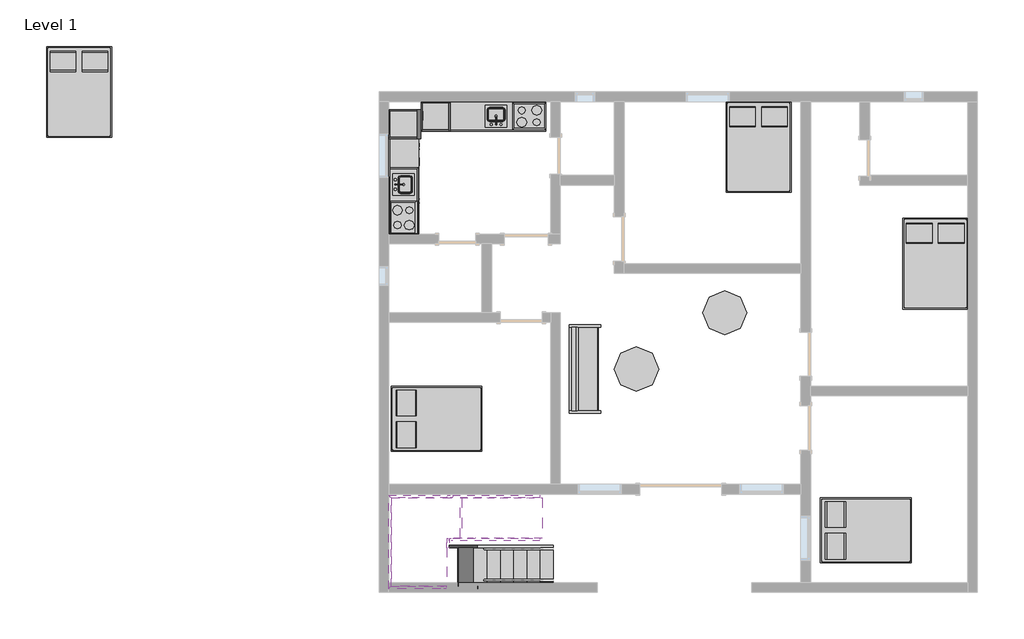
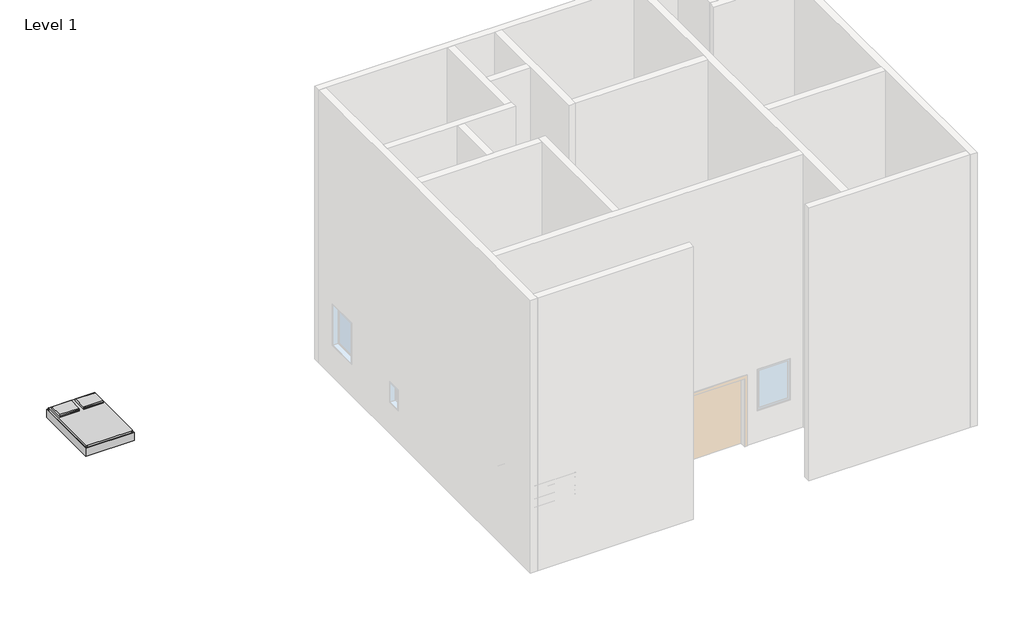
# One storey, part 4 of 4: 10 furniture elements, 8 members, 8 proxies, 2 flow terminals, 2 stair flights, 1 slab.
"""IFC4 building model written with IfcOpenShell, lengths in millimetres."""

from ifc_helpers import new_model, si_unit, frame, origin, place, context, project, spatial, polyline, outline, extrude, faceted_brep, transform, mapped, element, save
from components import m_cook_top_4_unit2_0615_x_500mm_249f3515, m_dishwasher_610_x_610_x_875mm_54ecfc4c, m_kitchenette_medium_1372mm_e05c6bec, m_refrigerator_600_x_660mm_a466bf94, m_sink_kitchen_island_450_x_450mm_f969cf2d, m_bed_box_1346_x_1880mm_double_b32eb57e, m_counter_top_w_sink_hole_600mm_depth_0a237b63, m_sofa_1830mm_f9e8a66b, m_table_dining_round_w_chairs_0915mm_diameter_5defa876, non_monolithic_landing_29a5f23a, stair_flight_50mm_tread_25mm_nosing_13mm_riser_b8c52427, stair_flight_50mm_tread_25mm_nosing_13mm_riser_89ce4123

model = new_model("IFC4")

# Units and contexts
model_context = context("Model", 3, world=origin())
ifc_project = project(units=[si_unit("LENGTHUNIT", "METRE", prefix="MILLI")], contexts=[model_context])

# Site, building, storey
site = spatial("IfcSite", under=ifc_project)
building = spatial("IfcBuilding", under=site)
storey = spatial("IfcBuildingStorey", under=building, Name="Level 1", Elevation=0.0)

# Proxies
placement = place(None, origin())
m_cook_top_4_unit2_0615_x_500mm_shape = m_cook_top_4_unit2_0615_x_500mm_249f3515(model_context)
element("IfcBuildingElementProxy", 1, Name="M_Cook Top-4 Unit2 : 0615 x 500mm", ObjectType="M_Cook Top-4 Unit2 : 0615 x 500mm", at=placement, inside=storey, context=model_context, shape_type="MappedRepresentation", body=[
    mapped(m_cook_top_4_unit2_0615_x_500mm_shape, transform((-10253.8870075, 9045.0865734, 0.0), x_axis=(0.0, 1.0, 0.0), y_axis=(-1.0, 0.0, 0.0), z_axis=(0.0, 0.0, 1.0))),
])
element("IfcBuildingElementProxy", 2, Name="M_Cook Top-4 Unit2 : 0615 x 500mm", ObjectType="M_Cook Top-4 Unit2 : 0615 x 500mm", at=placement, inside=storey, context=model_context, shape_type="MappedRepresentation", body=[
    mapped(m_cook_top_4_unit2_0615_x_500mm_shape, transform((-7648.6870075, 11143.4865734, 0.0), x_axis=(-0.9999999999999998, 0.0, 0.0), y_axis=(0.0, -0.9999999999999998, 0.0), z_axis=(0.0, 0.0, 1.0))),
])
m_dishwasher_610_x_610_x_875mm_shape = m_dishwasher_610_x_610_x_875mm_54ecfc4c(model_context)
element("IfcBuildingElementProxy", 3, Name="M_Dishwasher : 610 x 610 x 875mm", ObjectType="M_Dishwasher : 610 x 610 x 875mm", at=placement, inside=storey, context=model_context, shape_type="MappedRepresentation", body=[
    mapped(m_dishwasher_610_x_610_x_875mm_shape, transform((-9987.2374428, 9994.5691049, 0.0), x_axis=(0.0, 1.0, 0.0), y_axis=(-1.0, 0.0, 0.0), z_axis=(0.0, 0.0, 1.0))),
])
element("IfcBuildingElementProxy", 4, Name="M_Dishwasher : 610 x 610 x 875mm", ObjectType="M_Dishwasher : 610 x 610 x 875mm", at=placement, inside=storey, context=model_context, shape_type="MappedRepresentation", body=[
    mapped(m_dishwasher_610_x_610_x_875mm_shape, transform((-8598.169539, 11410.1361382, 0.0), x_axis=(-0.9999999999999998, 0.0, 0.0), y_axis=(0.0, -0.9999999999999998, 0.0), z_axis=(0.0, 0.0, 1.0))),
])
m_kitchenette_medium_1372mm_shape = m_kitchenette_medium_1372mm_e05c6bec(model_context)
element("IfcBuildingElementProxy", 5, Name="M_Kitchenette - Medium : 1372mm", ObjectType="M_Kitchenette - Medium : 1372mm", at=placement, inside=storey, context=model_context, shape_type="MappedRepresentation", body=[
    mapped(m_kitchenette_medium_1372mm_shape, transform((-10558.8870075, 9369.3488685, 0.0), x_axis=(0.0, 1.0, 0.0), y_axis=(-1.0, 0.0, 0.0), z_axis=(0.0, 0.0, 1.0))),
])
element("IfcBuildingElementProxy", 6, Name="M_Kitchenette - Medium : 1372mm", ObjectType="M_Kitchenette - Medium : 1372mm", at=placement, inside=storey, context=model_context, shape_type="MappedRepresentation", body=[
    mapped(m_kitchenette_medium_1372mm_shape, transform((-7972.9493026, 10838.4865734, 0.0), x_axis=(-0.9999999999999998, 0.0, 0.0), y_axis=(0.0, -0.9999999999999998, 0.0), z_axis=(0.0, 0.0, 1.0))),
])
m_refrigerator_600_x_660mm_shape = m_refrigerator_600_x_660mm_a466bf94(model_context)
element("IfcBuildingElementProxy", 7, Name="M_Refrigerator : 600 x 660mm", ObjectType="M_Refrigerator : 600 x 660mm", at=placement, inside=storey, context=model_context, shape_type="MappedRepresentation", body=[
    mapped(m_refrigerator_600_x_660mm_shape, transform((-10262.6719174, 11035.8877161, 0.0), x_axis=(0.0, 1.0, 0.0), y_axis=(-1.0, 0.0, 0.0), z_axis=(0.0, 0.0, 1.0))),
])
element("IfcBuildingElementProxy", 8, Name="M_Refrigerator : 600 x 660mm", ObjectType="M_Refrigerator : 600 x 660mm", at=placement, inside=storey, context=model_context, shape_type="MappedRepresentation", body=[
    mapped(m_refrigerator_600_x_660mm_shape, transform((-9639.4881502, 11134.7016636, 0.0), x_axis=(-0.9999999999999998, 0.0, 0.0), y_axis=(0.0, -0.9999999999999998, 0.0), z_axis=(0.0, 0.0, 1.0))),
])

# Flow terminals
m_sink_kitchen_island_450_x_450mm_shape = m_sink_kitchen_island_450_x_450mm_f969cf2d(model_context)
element("IfcFlowTerminal", 9, ObjectType="M_Sink Kitchen-Island : 450 x 450mm", at=placement, inside=storey, context=model_context, shape_type="MappedRepresentation", body=[
    mapped(m_sink_kitchen_island_450_x_450mm_shape, transform((-10251.5416064, 9715.3973329, 0.0), x_axis=(0.0, 1.0, 0.0), y_axis=(-1.0, 0.0, 0.0), z_axis=(0.0, 0.0, 1.0))),
])
element("IfcFlowTerminal", 10, ObjectType="M_Sink Kitchen-Island : 450 x 450mm", at=placement, inside=storey, context=model_context, shape_type="MappedRepresentation", body=[
    mapped(m_sink_kitchen_island_450_x_450mm_shape, transform((-8318.997767, 11145.8319745, 0.0), x_axis=(-0.9999999999999998, 0.0, 0.0), y_axis=(0.0, -0.9999999999999998, 0.0), z_axis=(0.0, 0.0, 1.0))),
])

# Furniture
m_bed_box_1346_x_1880mm_double_shape = m_bed_box_1346_x_1880mm_double_b32eb57e(model_context)
element("IfcFurniture", 11, ObjectType="M_Bed-Box : 1346 x 1880mm - Double", at=placement, inside=storey, context=model_context, shape_type="MappedRepresentation", body=[
    mapped(m_bed_box_1346_x_1880mm_double_shape, transform((-3239.8394666, 10742.9160816, 0.0), x_axis=(1.0, 0.0, 0.0), y_axis=(0.0, 1.0, 0.0), z_axis=(0.0, 0.0, 1.0))),
])
element("IfcFurniture", 12, ObjectType="M_Bed-Box : 1346 x 1880mm - Double", at=placement, inside=storey, context=model_context, shape_type="MappedRepresentation", body=[
    mapped(m_bed_box_1346_x_1880mm_double_shape, transform((-17309.8394666, 11882.9160816, 0.0), x_axis=(1.0, 0.0, 0.0), y_axis=(0.0, 1.0, 0.0), z_axis=(0.0, 0.0, 1.0))),
])
element("IfcFurniture", 13, ObjectType="M_Bed-Box : 1346 x 1880mm - Double", at=placement, inside=storey, context=model_context, shape_type="MappedRepresentation", body=[
    mapped(m_bed_box_1346_x_1880mm_double_shape, transform((420.9605334, 8326.9160816, 0.0), x_axis=(1.0, 0.0, 0.0), y_axis=(0.0, 1.0, 0.0), z_axis=(0.0, 0.0, 1.0))),
])
element("IfcFurniture", 14, ObjectType="M_Bed-Box : 1346 x 1880mm - Double", at=placement, inside=storey, context=model_context, shape_type="MappedRepresentation", body=[
    mapped(m_bed_box_1346_x_1880mm_double_shape, transform((-912.5165157, 2230.5341144, 0.0), x_axis=(0.0, 1.0000000000000007, 0.0), y_axis=(-1.0000000000000007, 0.0, 0.0), z_axis=(0.0, 0.0, 1.0))),
])
element("IfcFurniture", 15, ObjectType="M_Bed-Box : 1346 x 1880mm - Double", at=placement, inside=storey, context=model_context, shape_type="MappedRepresentation", body=[
    mapped(m_bed_box_1346_x_1880mm_double_shape, transform((-9801.3165157, 4540.3341144, 0.0), x_axis=(0.0, 1.0, 0.0), y_axis=(-1.0, 0.0, 0.0), z_axis=(0.0, 0.0, 1.0))),
])
m_counter_top_w_sink_hole_600mm_depth_shape = m_counter_top_w_sink_hole_600mm_depth_0a237b63(model_context)
element("IfcFurniture", 16, ObjectType="M_Counter Top w Sink Hole : 600mm Depth", at=placement, inside=storey, context=model_context, shape_type="MappedRepresentation", body=[
    mapped(m_counter_top_w_sink_hole_600mm_depth_shape, transform((-10558.8870075, 9902.5488685, 0.0), x_axis=(0.0, 1.0, 0.0), y_axis=(-1.0, 0.0, 0.0), z_axis=(0.0, 0.0, 1.0))),
])
element("IfcFurniture", 17, ObjectType="M_Counter Top w Sink Hole : 600mm Depth", at=placement, inside=storey, context=model_context, shape_type="MappedRepresentation", body=[
    mapped(m_counter_top_w_sink_hole_600mm_depth_shape, transform((-8506.1493026, 10838.4865734, 0.0), x_axis=(-0.9999999999999998, 0.0, 0.0), y_axis=(0.0, -0.9999999999999998, 0.0), z_axis=(0.0, 0.0, 1.0))),
])
m_sofa_1830mm_shape = m_sofa_1830mm_f9e8a66b(model_context)
element("IfcFurniture", 18, ObjectType="M_Sofa : 1830mm", at=placement, inside=storey, context=model_context, shape_type="MappedRepresentation", body=[
    mapped(m_sofa_1830mm_shape, transform((-6347.1329092, 5839.3160816, 0.0), x_axis=(0.0, 1.0000000000000002, 0.0), y_axis=(-1.0000000000000002, 0.0, 0.0), z_axis=(0.0, 0.0, 1.0))),
])
m_table_dining_round_w_chairs_0915mm_diameter_shape = m_table_dining_round_w_chairs_0915mm_diameter_5defa876(model_context)
element("IfcFurniture", 19, ObjectType="M_Table-Dining Round : 0915mm Diameter", at=placement, inside=storey, context=model_context, shape_type="MappedRepresentation", body=[
    mapped(m_table_dining_round_w_chairs_0915mm_diameter_shape, transform((-5531.7689748, 6094.5652619, 0.0), x_axis=(1.0, 0.0, 0.0), y_axis=(0.0, 1.0, 0.0), z_axis=(0.0, 0.0, 1.0))),
])
element("IfcFurniture", 20, ObjectType="M_Table-Dining Round w Chairs : 0915mm Diameter", at=placement, inside=storey, context=model_context, shape_type="MappedRepresentation", body=[
    mapped(m_table_dining_round_w_chairs_0915mm_diameter_shape, transform((-3702.9689748, 7261.3652619, 0.0), x_axis=(1.0, 0.0, 0.0), y_axis=(0.0, 1.0, 0.0), z_axis=(0.0, 0.0, 1.0))),
])

# Members
element("IfcMember", 21, ObjectType="Stringer - 50mm Width", at=placement, inside=storey, context=model_context, shape_type="SweptSolid", body=[
    extrude(outline(polyline([(0.0, -7153.6870075), (215.089535, -7153.6870075), (1612.6111183, -9363.5180111), (1212.6111183, -9479.3870711), (0.0, -7561.9457404), (0.0, -7153.6870075)])), frame((0.0, 1362.2865734, 0.0), z_axis=(0.0, 1.0, 0.0), x_axis=(0.0, 0.0, 1.0)), (0.0, 0.0, 1.0), 50.0),
])
element("IfcMember", 22, ObjectType="Stringer - 50mm Width", at=placement, inside=storey, context=model_context, shape_type="SweptSolid", body=[
    extrude(outline(polyline([(0.0, -7153.6870075), (215.089535, -7153.6870075), (1574.7733295, -9303.6870075), (1101.4964536, -9303.6870075), (0.0, -7561.9457404), (0.0, -7153.6870075)])), frame((0.0, 2212.3123547, 0.0), z_axis=(0.0, 1.0, 0.0), x_axis=(0.0, 0.0, 1.0)), (0.0, 0.0, 1.0), 50.0),
])
element("IfcMember", 23, ObjectType="Stringer - 50mm Width", at=placement, inside=storey, context=model_context, shape_type="SweptSolid", body=[
    extrude(outline(polyline([(1612.6111183, -9343.856004), (1212.6111183, -9227.986944), (2350.5083113, -7428.6870075), (2823.7851872, -7428.6870075), (1612.6111183, -9343.856004)])), frame((0.0, 3244.2865734, 0.0), z_axis=(0.0, 1.0, 0.0), x_axis=(0.0, 0.0, 1.0)), (0.0, 0.0, 1.0), 50.0),
])
element("IfcMember", 24, ObjectType="Stringer - 50mm Width", at=placement, inside=storey, context=model_context, shape_type="SweptSolid", body=[
    extrude(outline(polyline([(1638.0144362, -9303.6870075), (1212.6111183, -9303.6870075), (1212.6111183, -9227.986944), (2350.5083113, -7428.6870075), (2823.7851872, -7428.6870075), (1638.0144362, -9303.6870075)])), frame((0.0, 2358.8252453, 0.0), z_axis=(0.0, 1.0, 0.0), x_axis=(0.0, 0.0, 1.0)), (0.0, 0.0, 1.0), 50.0),
])
element("IfcMember", 25, ObjectType="Stringer - 50mm Width", at=placement, inside=storey, context=model_context, shape_type="Brep", body=[
    faceted_brep([(-9343.856004, 3244.2865734, 1612.6111183), (-9343.856004, 3294.2865734, 1612.6111183), (-10558.0870075, 3294.2865734, 1612.6111183), (-10508.0870075, 3244.2865734, 1612.6111183), (-9227.986944, 3244.2865734, 1212.6111183), (-10508.0870075, 3244.2865734, 1212.6111183), (-9227.986944, 3294.2865734, 1212.6111183), (-10558.0870075, 3294.2865734, 1212.6111183)], [[[0, 1, 2, 3]], [[4, 0, 3, 5]], [[6, 4, 5, 7]], [[1, 6, 7, 2]], [[1, 0, 4, 6]], [[2, 7, 5, 3]]]),
])
element("IfcMember", 26, ObjectType="Stringer - 50mm Width", at=placement, inside=storey, context=model_context, shape_type="SweptSolid", body=[
    extrude(outline(polyline([(-10558.0870075, 3294.2865734), (-10508.0870075, 3244.2865734), (-10508.0870075, 1412.2865734), (-10558.0870075, 1362.2865734), (-10558.0870075, 3294.2865734)])), frame((0.0, 0.0, 1212.6111183), z_axis=(0.0, 0.0, 1.0), x_axis=(1.0, 0.0, 0.0)), (0.0, 0.0, 1.0), 400.0),
])
element("IfcMember", 27, ObjectType="Stringer - 50mm Width", at=placement, inside=storey, context=model_context, shape_type="Brep", body=[
    faceted_brep([(-10508.0870075, 1412.2865734, 1612.6111183), (-10558.0870075, 1362.2865734, 1612.6111183), (-9363.5180111, 1362.2865734, 1612.6111183), (-9363.5180111, 1412.2865734, 1612.6111183), (-10508.0870075, 1412.2865734, 1212.6111183), (-9479.3870711, 1412.2865734, 1212.6111183), (-10558.0870075, 1362.2865734, 1212.6111183), (-9479.3870711, 1362.2865734, 1212.6111183)], [[[0, 1, 2, 3]], [[4, 0, 3, 5]], [[6, 4, 5, 7]], [[1, 6, 7, 2]], [[1, 0, 4, 6]], [[2, 7, 5, 3]]]),
])
element("IfcMember", 28, ObjectType="Stringer - 50mm Width", at=placement, inside=storey, context=model_context, shape_type="SweptSolid", body=[
    extrude(outline(polyline([(-9303.6870075, 2212.3123547), (-9353.6870075, 2212.3123547), (-9353.6870075, 2408.8252453), (-9303.6870075, 2408.8252453), (-9303.6870075, 2212.3123547)])), frame((0.0, 0.0, 1212.6111183), z_axis=(0.0, 0.0, 1.0), x_axis=(1.0, 0.0, 0.0)), (0.0, 0.0, 1.0), 400.0),
])

# Slab
non_monolithic_landing_shape = non_monolithic_landing_29a5f23a(model_context)
element("IfcSlab", 29, ObjectType="Non-Monolithic Landing", at=placement, inside=storey, context=model_context, shape_type="MappedRepresentation", body=[
    mapped(non_monolithic_landing_shape, transform((0.0, 0.0, 0.0), x_axis=(1.0, 0.0, 0.0), y_axis=(0.0, 1.0, 0.0), z_axis=(0.0, 0.0, 1.0))),
])

# Stair flights
stair_flight_50mm_tread_25mm_nosing_13mm_riser_shape = stair_flight_50mm_tread_25mm_nosing_13mm_riser_b8c52427(model_context)
element("IfcStairFlight", 30, ObjectType="50mm Tread 25mm Nosing 13mm Riser", at=placement, inside=storey, context=model_context, shape_type="MappedRepresentation", body=[
    mapped(stair_flight_50mm_tread_25mm_nosing_13mm_riser_shape, transform((0.0, 0.0, 0.0), x_axis=(1.0, 0.0, 0.0), y_axis=(0.0, 1.0, 0.0), z_axis=(0.0, 0.0, 1.0))),
])
stair_flight_50mm_tread_25mm_nosing_13mm_riser_2_shape = stair_flight_50mm_tread_25mm_nosing_13mm_riser_89ce4123(model_context)
element("IfcStairFlight", 31, ObjectType="50mm Tread 25mm Nosing 13mm Riser", at=placement, inside=storey, context=model_context, shape_type="MappedRepresentation", body=[
    mapped(stair_flight_50mm_tread_25mm_nosing_13mm_riser_2_shape, transform((0.0, 0.0, 0.0), x_axis=(1.0, 0.0, 0.0), y_axis=(0.0, 1.0, 0.0), z_axis=(0.0, 0.0, 1.0))),
])

save(model, "model.ifc")

# Revit data of these elements
# Type "M_Cook Top-4 Unit2 : 0615 x 500mm"
#   Depth = 500 mm
#   Width = 615 mm
#   Burner Material = Steel, Chrome Plated
#   Cooktop Material = Steel, Polished
#   Default Elevation = 0
#   Assembly Code = ""
# Type "M_Dishwasher : 610 x 610 x 875mm"
#   Label = "DW"
#   Depth = 610 mm
#   Height = 875 mm
#   Width = 610 mm
#   Dishwasher Material = Steel, Paint Finish, Ivory, Glossy
#   Panel Face Material = Plastic, Opaque Black
#   Default Elevation = 0
# Type "M_Kitchenette - Medium : 1372mm"
#   Counter Length = 1980 mm
#   Cabinet Width = 1372 mm
#   Cabinet Height = 900 mm
#   Cabinet Depth = 610 mm
#   Toe Depth = 35 mm
#   Toe Height = 100 mm
#   Cabinet Material = Cabinets
#   Door/Drawer Material = Cabinets
#   Handle Material = Cabinets - Handles
#   Default Elevation = 0
# Type "M_Refrigerator : 600 x 660mm"
#   Label = "REF."
#   Depth = 660 mm
#   Height = 1830 mm
#   Width = 600 mm
#   Material = Steel, Paint Finish, Ivory, Matte
#   Description = (empty or 0)
#   Default Elevation = 0
# Type "M_Sink Kitchen-Island : 450 x 450mm"
#   Counter Height [instance default] = 900 mm
#   Depth = 450 mm
#   Width = 450 mm
#   Fixture Material = Steel, Polished
#   Sink Material = Steel, Polished
#   Default Elevation = 0
# Type "M_Bed-Box : 1346 x 1880mm - Double"
#   Length = 1880 mm
#   Width = 1346 mm
#   Frame Material = Birch
#   Mattress Material = Linen, White
#   Default Elevation = 0
# Type "M_Counter Top w Sink Hole : 600mm Depth"
#   Counter Thickness = 40 mm
#   Depth = 625 mm
#   Height = 900 mm
#   Length [instance default] = 2500 mm
#   Sink Location [instance default] = 1200 mm
#   Sink Location To Wall [instance default] = 100 mm
#   Sink Opening Depth [instance default] = 378 mm
#   Sink Opening Width [instance default] = 587 mm
#   Counter Top Material = none
#   Default Elevation = 0
# Type "M_Sofa : 1830mm"
#   Width = 1830 mm
#   Seat Material = Linen, Beige
#   Frame Material = Cherry
#   Default Elevation = 0
# Type "M_Table-Dining Round : 0915mm Diameter"
#   Diameter = 915 mm
#   Height = 762 mm
#   Base Material = Pine
#   Top Material = Laminate, Linen, Matte
#   Default Elevation = 0
# Type "M_Table-Dining Round w Chairs : 0915mm Diameter"
#   Radius = 457.5 mm
#   Diameter = 915 mm
#   Height = 762 mm
#   Chairs = 4
#   Base Material = Pine
#   Top Material = Laminate, Linen, Matte
#   Default Elevation = 0
# Elements 1, 2 (IfcBuildingElementProxy, "M_Cook Top-4 Unit2 : 0615 x 500mm")
#   Phase Created = New Construction
#   Materials on its faces: "Steel, Polished", "Steel, Chrome Plated"
# Elements 3, 4 (IfcBuildingElementProxy, "M_Dishwasher : 610 x 610 x 875mm")
#   Phase Created = New Construction
#   Materials on its faces: "Steel, Paint Finish, Ivory, Glossy", "Plastic, Opaque Black"
# Elements 5, 6 (IfcBuildingElementProxy, "M_Kitchenette - Medium : 1372mm")
#   Phase Created = New Construction
#   Materials on its faces: "Cabinets", "Cabinets - Handles"
# Elements 7, 8 (IfcBuildingElementProxy, "M_Refrigerator : 600 x 660mm")
#   Phase Created = New Construction
#   Materials on its faces: "Steel, Paint Finish, Ivory, Matte", "Steel, Chrome Plated"
# Element 9 (IfcFlowTerminal, "M_Sink Kitchen-Island : 450 x 450mm")
#   Mark = "1"
#   Counter Height = 900 mm
#   Phase Created = New Construction
#   Materials on its faces: "Steel, Polished"
# Element 10 (IfcFlowTerminal, "M_Sink Kitchen-Island : 450 x 450mm")
#   Mark = "2"
#   Counter Height = 900 mm
#   Phase Created = New Construction
#   Materials on its faces: "Steel, Polished"
# Elements 11, 12, 13, 14, 15 (IfcFurniture, "M_Bed-Box : 1346 x 1880mm - Double")
#   Phase Created = New Construction
#   Materials on its faces: "Birch", "Linen, White"
# Elements 16, 17 (IfcFurniture, "M_Counter Top w Sink Hole : 600mm Depth")
#   Sink Opening Width = 400 mm
#   Sink Opening Depth = 350 mm
#   Sink Location To Wall = 160 mm
#   Sink Location = 1025 mm
#   Length = 1980 mm
#   Phase Created = New Construction
#   Materials on its faces: "Counter Top"
# Element 18 (IfcFurniture, "M_Sofa : 1830mm")
#   Phase Created = New Construction
#   Materials on its faces: "Cherry", "Linen, Beige"
# Element 19 (IfcFurniture, "M_Table-Dining Round : 0915mm Diameter")
#   Phase Created = New Construction
#   Materials on its faces: "Pine", "Laminate, Linen, Matte"
# Element 20 (IfcFurniture, "M_Table-Dining Round w Chairs : 0915mm Diameter")
#   Phase Created = New Construction
#   Materials on its faces: "Pine", "Laminate, Linen, Matte"
# Elements 21, 22, 23, 24, 25, 26, 27, 28 (IfcMember, "Stringer - 50mm Width")
#   Phase Created = New Construction
# Element 29 (IfcSlab, "Non-Monolithic Landing")
#   Phase Created = New Construction
# Elements 30, 31 (IfcStairFlight, "50mm Tread 25mm Nosing 13mm Riser")
#   Phase Created = New Construction
# Materials
#   "Steel, Chrome Plated": class "Metal", colour RGB 244 244 244, transparency 0, Description = "Chromiuim plated steel", Cost = 0
#   "Steel, Polished": class "Metal", colour RGB 57 57 57, transparency 0, Description = "Polished steel", Cost = 0
#   "Steel, Paint Finish, Ivory, Glossy": class "Metal", colour RGB 247 247 239, transparency 0, Description = "Steel, paint finish, ivory, glossy", Cost = 0
#   "Plastic, Opaque Black": class "Plastic", colour RGB 0 0 0, transparency 0.7, Description = "Plastic, generic, opaque black", Cost = 0
#   "Cabinets": colour RGB 249 249 249, transparency 0
#   "Cabinets - Handles": class "Metal", colour RGB 57 57 57, transparency 0
#   "Steel, Paint Finish, Ivory, Matte": class "Metal", colour RGB 247 247 239, transparency 0, Description = "Steel, paint finish, ivory, matte", Cost = 0
#   "Birch": class "Wood", colour RGB 224 178 126, transparency 0, Description = "Betula Alleghaniensis", Cost = 0
#   "Linen, White": class "Textile", colour RGB 247 247 239, transparency 0, Description = "Linen, white", Cost = 0
#   "Linen, Beige": class "Textile", colour RGB 249 239 230, transparency 0, Description = "Linen, beige", Cost = 0
#   "Cherry": class "Wood", colour RGB 154 107 61, transparency 0, Description = "Prunus Serotina", Cost = 0
#   "Pine": class "Wood", colour RGB 223 192 134, transparency 0, Description = "Pinus Echinata", Cost = 0
#   "Laminate, Linen, Matte": class "Plastic", colour RGB 249 239 230, transparency 0, Description = "Plastic Laminate - Linen, Matte", Cost = 0
#   "Counter Top": class "Wood", colour RGB 226 177 128, transparency 0
